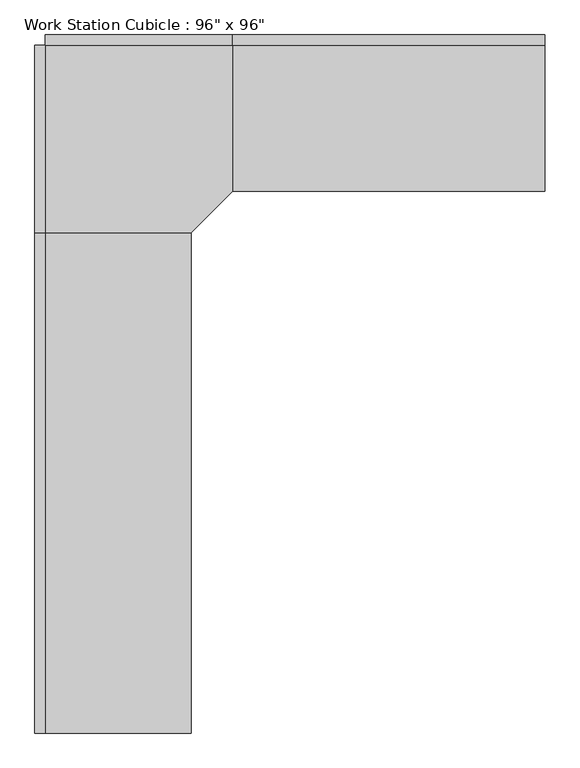
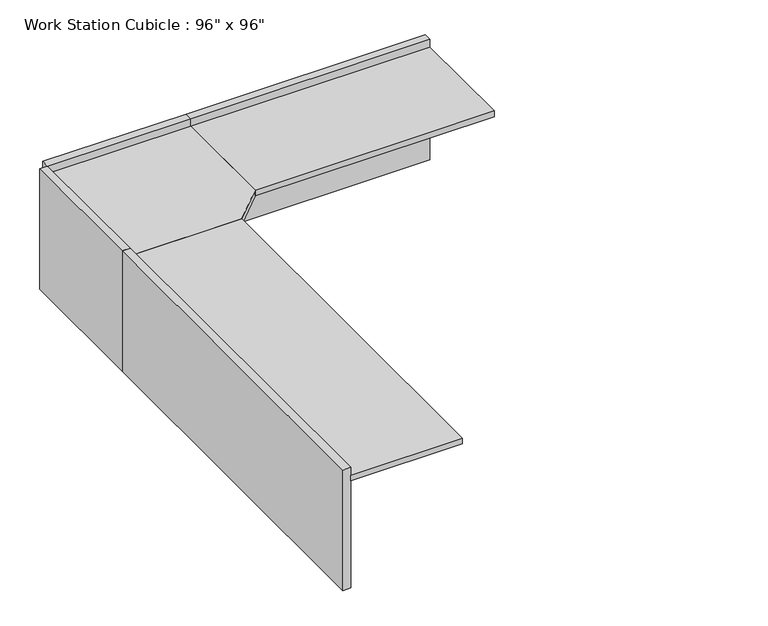
"""IFC4 building model written with IfcOpenShell, lengths in millimetres: furniture geometry."""

from ifc_helpers import new_model, si_unit, frame, origin, origin_with_axes, place, context, project, spatial, polyline, outline, extrude, source, transform, mapped, element, save


def furniture_f7403a93(model_context):
    return source(origin(), model_context, "Body", "SweptSolid", [
        extrude(outline(polyline([(-80.9317522, -545.8230076), (833.4682478, -545.8230076), (833.4682478, -1257.0230076), (630.2682478, -1460.2230076), (-80.9317522, -1460.2230076), (-80.9317522, -545.8230076)])), frame((0.0, 0.0, 723.9), z_axis=(0.0, 0.0, 1.0), x_axis=(1.0, 0.0, 0.0)), (0.0, 0.0, 1.0), 38.1),
        extrude(outline(polyline([(630.2682478, -3898.6230076), (-80.9317522, -3898.6230076), (-80.9317522, -1460.2230076), (630.2682478, -1460.2230076), (630.2682478, -3898.6230076)])), frame((0.0, 0.0, 723.9), z_axis=(0.0, 0.0, 1.0), x_axis=(1.0, 0.0, 0.0)), (0.0, 0.0, 1.0), 38.1),
        extrude(outline(polyline([(2357.4682478, -1257.0230076), (833.4682478, -1257.0230076), (833.4682478, -545.8230076), (2357.4682478, -545.8230076), (2357.4682478, -1257.0230076)])), frame((0.0, 0.0, 723.9), z_axis=(0.0, 0.0, 1.0), x_axis=(1.0, 0.0, 0.0)), (0.0, 0.0, 1.0), 38.1),
        extrude(outline(polyline([(2357.4682478, -545.8230076), (833.4682478, -545.8230076), (833.4682478, -495.0230076), (2357.4682478, -495.0230076), (2357.4682478, -545.8230076)])), origin_with_axes(), (0.0, 0.0, 1.0), 812.8),
        extrude(outline(polyline([(833.4682478, -545.8230076), (-80.9317522, -545.8230076), (-80.9317522, -495.0230076), (833.4682478, -495.0230076), (833.4682478, -545.8230076)])), origin_with_axes(), (0.0, 0.0, 1.0), 812.8),
        extrude(outline(polyline([(-80.9317522, -1460.2230076), (-131.7317522, -1460.2230076), (-131.7317522, -545.8230076), (-80.9317522, -545.8230076), (-80.9317522, -1460.2230076)])), origin_with_axes(), (0.0, 0.0, 1.0), 812.8),
        extrude(outline(polyline([(-80.9317522, -3898.6230076), (-131.7317522, -3898.6230076), (-131.7317522, -1460.2230076), (-80.9317522, -1460.2230076), (-80.9317522, -3898.6230076)])), origin_with_axes(), (0.0, 0.0, 1.0), 812.8),
    ])


if __name__ == "__main__":
    model = new_model("IFC4")
    model_context = context("Model", 3, world=origin())
    ifc_project = project(units=[si_unit("LENGTHUNIT", "METRE", prefix="MILLI")], contexts=[model_context])
    site = spatial("IfcSite", under=ifc_project)
    building = spatial("IfcBuilding", under=site)
    placement = place(None, origin())
    furniture_shape = furniture_f7403a93(model_context)
    element("IfcFurniture", 1, ObjectType="Work Station Cubicle : 96\" x 96\"", at=placement, inside=building, context=model_context, shape_type="MappedRepresentation", body=[
        mapped(furniture_shape, transform((0.0, 0.0, 0.0), x_axis=(1.0, 0.0, 0.0), y_axis=(0.0, 1.0, 0.0), z_axis=(0.0, 0.0, 1.0))),
    ])
    save(model, "model.ifc")

# Revit data of these elements
# Type "Work Station Cubicle : 96\" x 96\""
#   Assembly Code = "E2020"
#   Desktop Height = 2' - 6"
#   Desktop1 Width = 2' - 4"
#   Desktop2 Width = 2' - 4"
#   Panel Height = 2' - 8"
#   Panel1 Length = 8' - 0"
#   Panel2 Length = 5' - 0"
#   Cube Panel Material = Textile - Light Gray
#   Work Top Material = Laminate, Ivory, Matte
#   Default Elevation = 0
# Element 1 (IfcFurniture, "Work Station Cubicle : 96\" x 96\"")
#   Materials on its faces: "Textile - Light Gray", "Laminate, Ivory, Matte"
# Materials
#   "Textile - Light Gray": class "Fabric", colour RGB 204 204 204, transparency 0
#   "Laminate, Ivory, Matte": class "Plastic", colour RGB 247 247 239, transparency 0, Description = "Plastic Laminate - Ivory, Matte", Cost = 0
